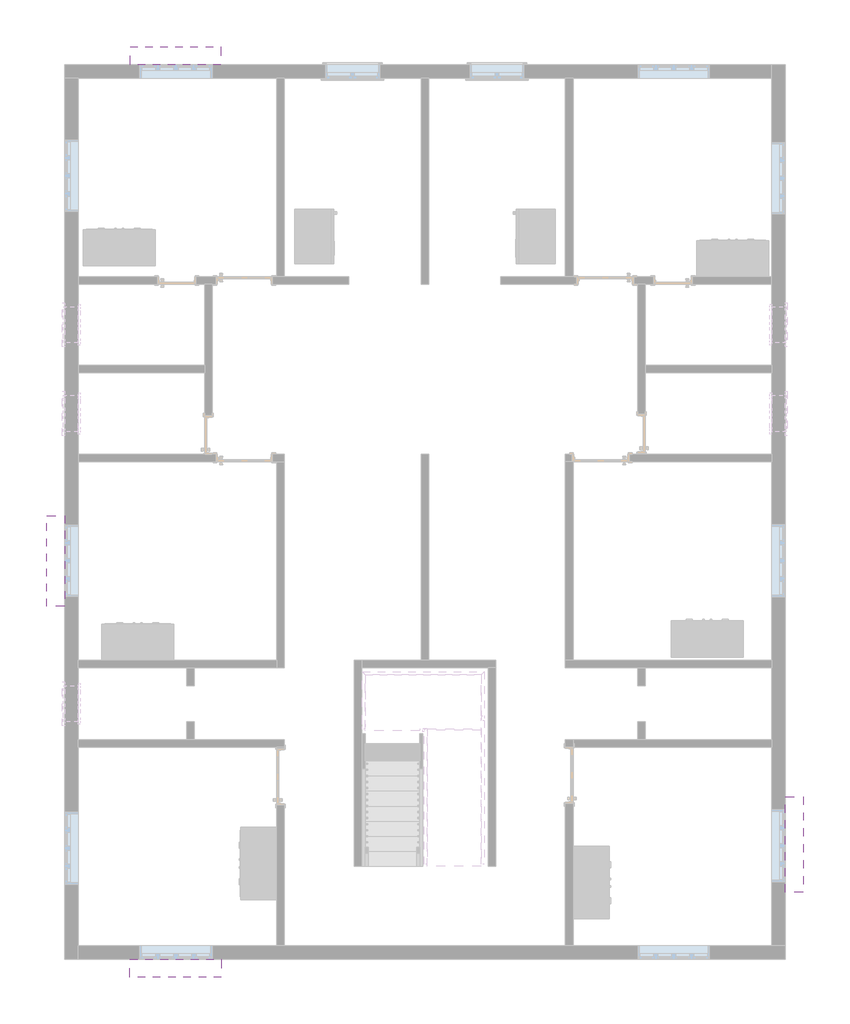
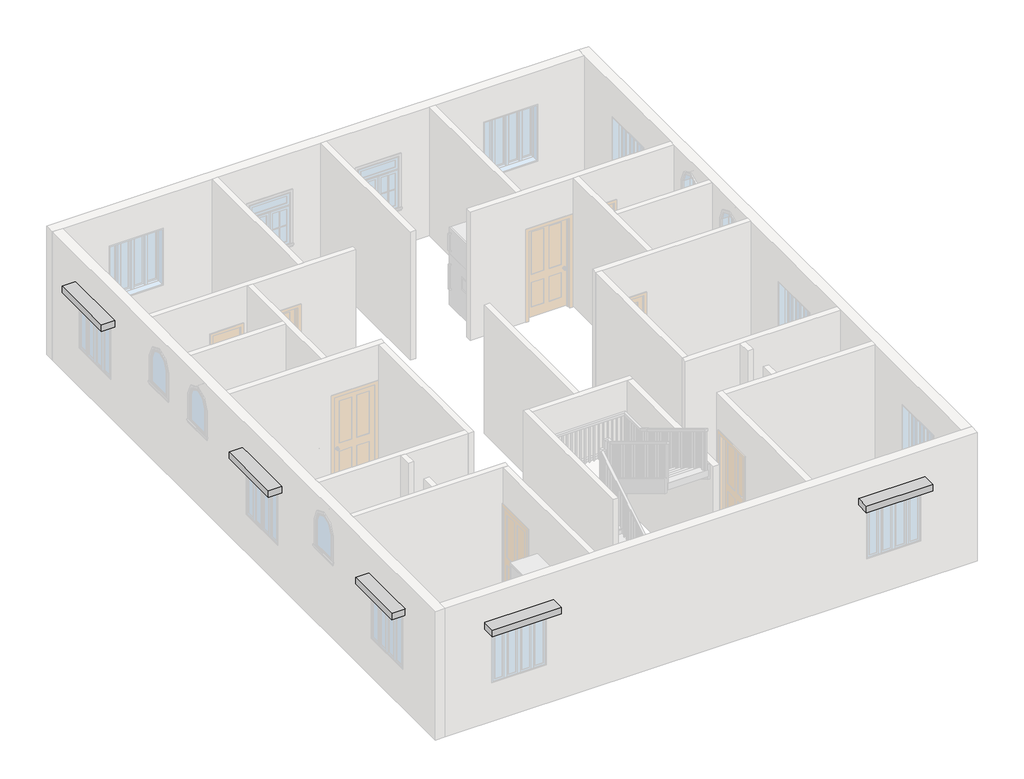
# One storey, part 4 of 4: 4 proxies.
"""IFC4 building model written with IfcOpenShell, lengths in millimetres."""

from ifc_helpers import new_model, si_unit, origin, place, context, project, spatial, transform, mapped, element, save
from components import generic_models_5_generic_models_1_03e322a7, generic_models_6_generic_models_2_9348183e, generic_models_7_generic_models_3_e4b45389, generic_models_8_generic_models_4_251d3b20

model = new_model("IFC4")

# Units and contexts
model_context = context("Model", 3, world=origin())
ifc_project = project(units=[si_unit("LENGTHUNIT", "METRE", prefix="MILLI")], contexts=[model_context])

# Site, building, storey
site = spatial("IfcSite", under=ifc_project)
building = spatial("IfcBuilding", under=site)
storey = spatial("IfcBuildingStorey", under=building, Elevation=3352.8)

# Proxies
placement = place(None, origin())
generic_models_5_generic_models_1_shape = generic_models_5_generic_models_1_03e322a7(model_context)
element("IfcBuildingElementProxy", 1, Name="Generic Models 5 : Generic Models 1", ObjectType="Generic Models 5 : Generic Models 1", at=placement, inside=storey, context=model_context, shape_type="MappedRepresentation", body=[
    mapped(generic_models_5_generic_models_1_shape, transform((0.0, 0.0, 0.0), x_axis=(1.0, 0.0, 0.0), y_axis=(0.0, 1.0, 0.0), z_axis=(0.0, 0.0, 1.0))),
])
generic_models_6_generic_models_2_shape = generic_models_6_generic_models_2_9348183e(model_context)
element("IfcBuildingElementProxy", 2, Name="Generic Models 6 : Generic Models 2", ObjectType="Generic Models 6 : Generic Models 2", at=placement, inside=storey, context=model_context, shape_type="MappedRepresentation", body=[
    mapped(generic_models_6_generic_models_2_shape, transform((0.0, 0.0, 0.0), x_axis=(1.0, 0.0, 0.0), y_axis=(0.0, 1.0, 0.0), z_axis=(0.0, 0.0, 1.0))),
])
generic_models_7_generic_models_3_shape = generic_models_7_generic_models_3_e4b45389(model_context)
element("IfcBuildingElementProxy", 3, Name="Generic Models 7 : Generic Models 3", ObjectType="Generic Models 7 : Generic Models 3", at=placement, inside=storey, context=model_context, shape_type="MappedRepresentation", body=[
    mapped(generic_models_7_generic_models_3_shape, transform((0.0, 0.0, 0.0), x_axis=(1.0, 0.0, 0.0), y_axis=(0.0, 1.0, 0.0), z_axis=(0.0, 0.0, 1.0))),
])
generic_models_8_generic_models_4_shape = generic_models_8_generic_models_4_251d3b20(model_context)
element("IfcBuildingElementProxy", 4, Name="Generic Models 8 : Generic Models 4", ObjectType="Generic Models 8 : Generic Models 4", at=placement, inside=storey, context=model_context, shape_type="MappedRepresentation", body=[
    mapped(generic_models_8_generic_models_4_shape, transform((0.0, 0.0, 0.0), x_axis=(1.0, 0.0, 0.0), y_axis=(0.0, 1.0, 0.0), z_axis=(0.0, 0.0, 1.0))),
])

save(model, "model.ifc")

# Revit data of these elements
# Element 1 (IfcBuildingElementProxy, "Generic Models 5 : Generic Models 1")
#   Phase Created = New Construction
# Element 2 (IfcBuildingElementProxy, "Generic Models 6 : Generic Models 2")
#   Phase Created = New Construction
# Element 3 (IfcBuildingElementProxy, "Generic Models 7 : Generic Models 3")
#   Phase Created = New Construction
# Element 4 (IfcBuildingElementProxy, "Generic Models 8 : Generic Models 4")
#   Phase Created = New Construction
